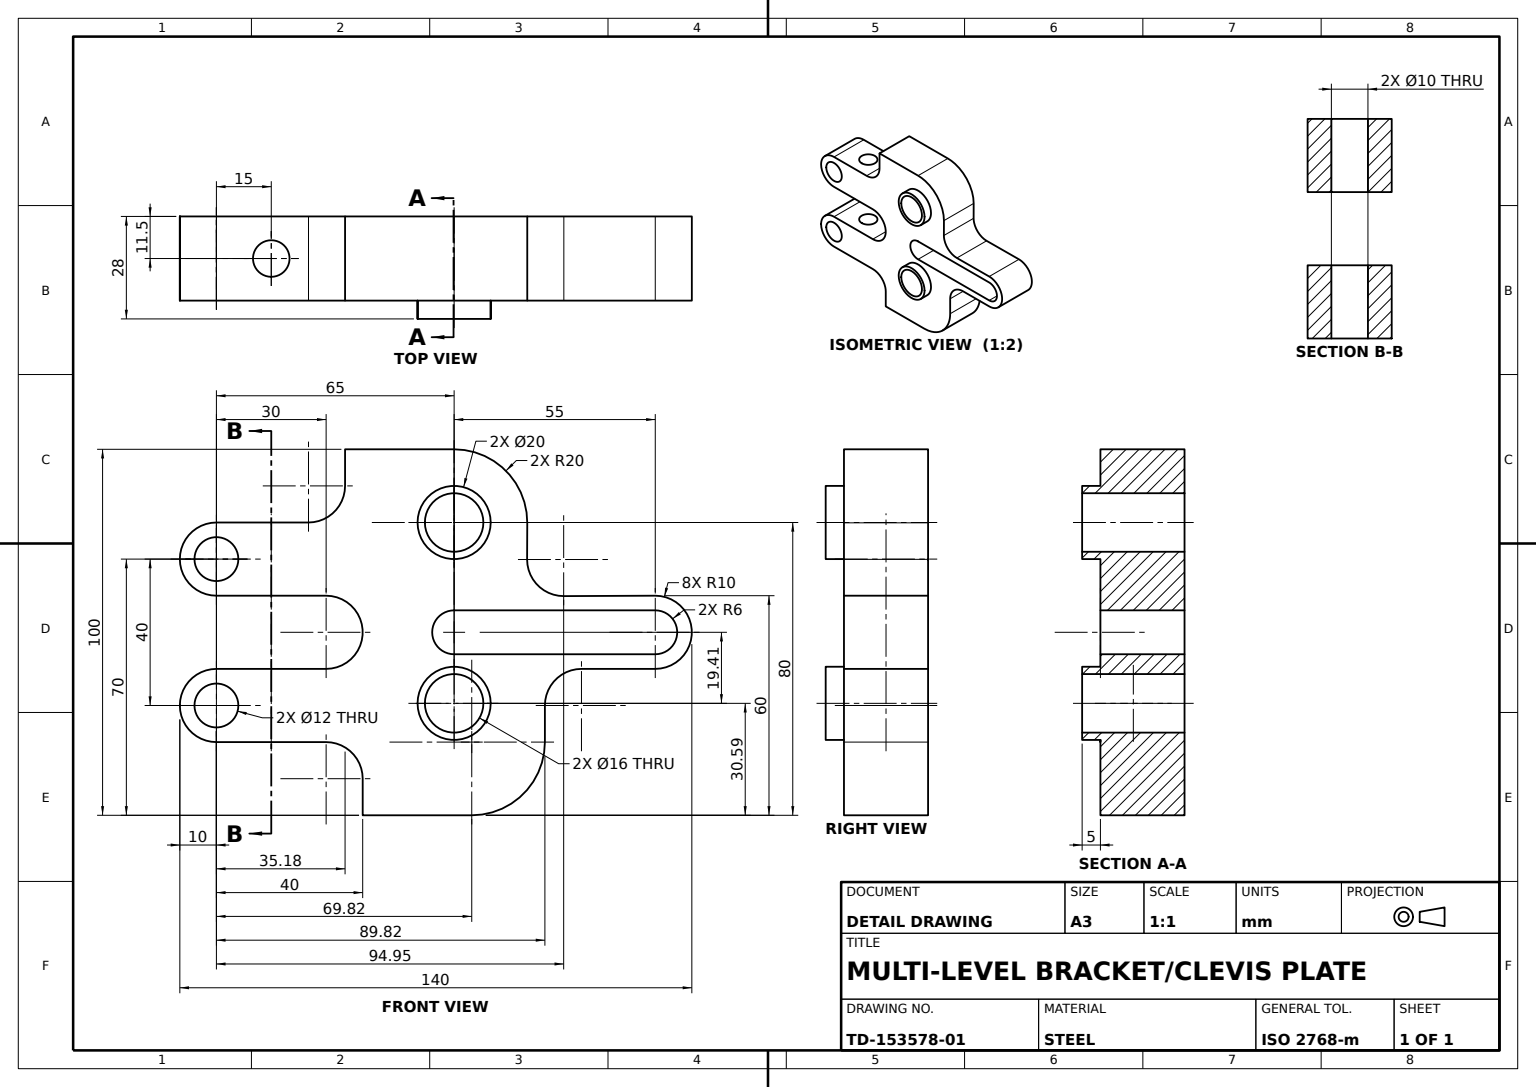
SolidWorks part; units mm, degrees
material "Plain Carbon Steel"
ref_plane "Front Plane" through (0, 0, 0) normal (0, 0, 1) x (1, 0, 0)
ref_plane "Top Plane" through (0, 0, 0) normal (0, 1, 0) x (1, 0, 0)
ref_plane "Right Plane" through (0, 0, 0) normal (1, 0, 0) x (0, 0, -1)
sketch "Bracket Profile Sketch" plane through (0, 0, 0) normal (0, 0, 1) x (1, 0, 0)
  line L0 (0, 0) -> (0, -20) construction
  line L1 (0, -20) -> (65, -20) construction
  line L2 (65, -20) -> (65, 30) construction
  line L3 (65, -20) -> (65, -70) construction
  line L4 (65, -20) -> (120, -20) construction
  line L5 (0, -20) -> (0, -40) construction
  line L6 (65, -70) -> (40, -70)
  line L7 (65, -70) -> (69.82, -70)
  line L8 (0, -50) -> (30, -50)
  line L9 (40, -60) -> (40, -70)
  line L10 (120, -30) -> (99.82, -30)
  line L11 (89.82, -40) -> (89.82, -50)
  line L12 (0, -20) -> (30, -20) construction
  line L13 (0, -10) -> (30, -10)
  line L14 (0, -30) -> (30, -30)
  line L15 (65, 30) -> (35.18, 30)
  line L16 (65, 30) -> (65.0002, 30)
  line L17 (0, 10) -> (25.18, 10)
  line L18 (35.18, 20) -> (35.18, 30)
  line L19 (120, -10) -> (95, -10.1125)
  line L20 (84.9551, -0.0676) -> (85, 9.91)
  line L21 (120, -20) -> (65, -20) construction
  line L22 (120, -26) -> (65, -26)
  line L23 (120, -14) -> (65, -14)
  circle A0 centre (0, 0) radius 6
  arc A1 (0, 10) -> (0, -10) centre (0, 0) ccw
  circle A2 centre (0, -40) radius 6
  arc A3 (0, -30) -> (0, -50) centre (0, -40) ccw
  arc A5 (120, -30) -> (120, -10) centre (120, -20) ccw
  arc A6 (40, -60) -> (30, -50) centre (30, -60) ccw
  arc A7 (99.82, -30) -> (89.82, -40) centre (99.82, -40) ccw
  arc A8 (89.82, -50) -> (69.82, -70) centre (69.82, -50) cw
  arc A9 (30, -30) -> (30, -10) centre (30, -20) ccw
  arc A10 (85, 9.91) -> (65.0002, 30) centre (65.0002, 10) ccw
  arc A11 (95, -10.1125) -> (84.9551, -0.0676) centre (94.955, -0.1126) cw
  arc A12 (35.18, 20) -> (25.18, 10) centre (25.18, 20) cw
  arc A13 (120, -26) -> (120, -14) centre (120, -20) ccw
  arc A14 (65, -14) -> (65, -26) centre (65, -20) ccw
  point P11 (92.5, -20)
  dimension "D1" = 12
  dimension "D2" = 20
  dimension "D3" = 12
  dimension "D4" = 20
  dimension "D6" = 6
  dimension "D7" = 20
  dimension "D8" = 10
  dimension "D9" = 10
  dimension "D10" = 20
  dimension "D11" = 20
  dimension "D12" = 30
  dimension "D18" = 20
  dimension "D19" = 10
  dimension "D26" = 20
  dimension "D5" = 40
  dimension "D13" = 30
  dimension "D14" = 70
  dimension "D15" = 40
  dimension "D16" = 65
  dimension "D17" = 100
  dimension "D20" = 55
  dimension "D21" = 35.18
  dimension "D22" = 69.82
  dimension "D23" = 59.91
  dimension "D24" = 120
  dimension "D25" = 95
  dimension "D27" = 0.1125
extrude "Bracket Base 23mm" add sketch "Bracket Profile Sketch" along normal blind 23
sketch "Boss Pad Sketch" plane through (0, 0, 23) normal (0, 0, 1) x (1, 0, 0)
  line L0 (65, -20) -> (120, -20) construction
  line L2 (30, -30) -> (0, -30) construction
  circle A0 centre (65, 10) radius 8
  circle A1 centre (65, 10) radius 10
  circle A2 centre (65, -39.4112) radius 8
  circle A3 centre (65, -39.4112) radius 10
  dimension "D1" = 16
  dimension "D2" = 20
  dimension "D5" = 20
  dimension "D6" = 16
  dimension "D3" = 65
  dimension "D4" = 30
  dimension "D7" = 9.4112
extrude "Boss Pad 5mm" add sketch "Boss Pad Sketch" along normal blind 5
sketch "Hole Ø10 Sketch" plane through (0, -50, 0) normal (0, -1, 0) x (1, 0, 0)
  line L0 (30, 23) -> (30, 0) construction
  line L1 (0, 0) -> (30, 0) construction
  circle A0 centre (15, 11.5) radius 5
  dimension "D1" = 10
  dimension "D2" = 15
  dimension "D3" = 11.5
extrude "Hole Ø10" cut sketch "Hole Ø10 Sketch" against normal through all
sketch "Profile Cut Sketch" plane through (0, 0, 23) normal (0, 0, 1) x (1, 0, 0)
  circle A0 centre (65, 10) radius 8
  circle A1 centre (65, -39.4112) radius 8
  dimension "D1" = 16
extrude "Profile Cut" cut sketch "Profile Cut Sketch" against normal through all
